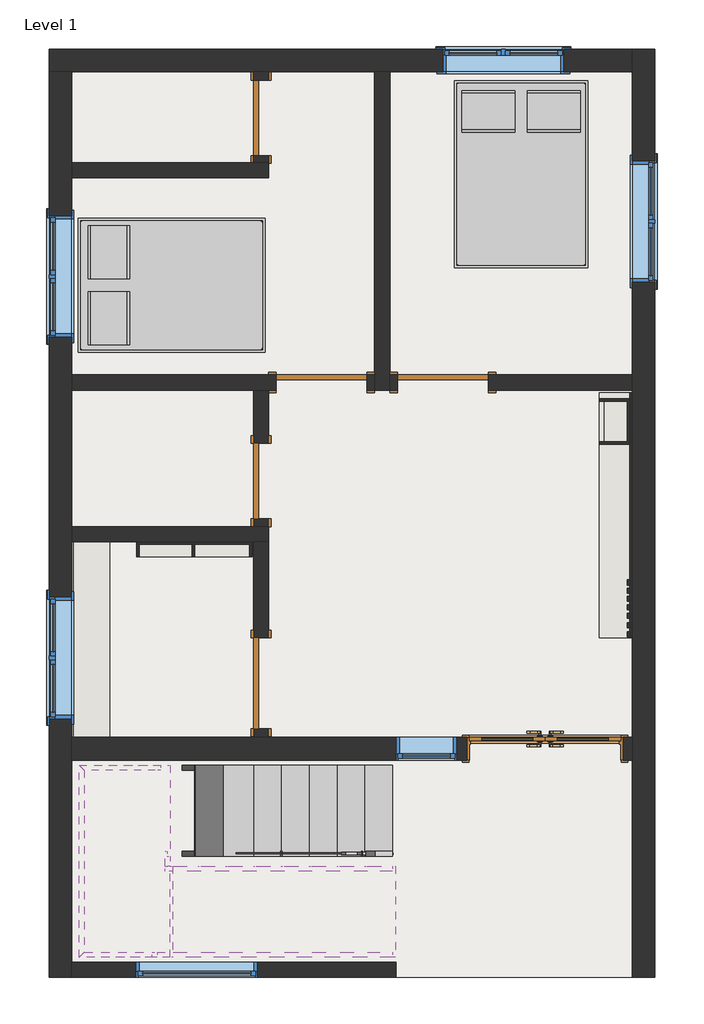
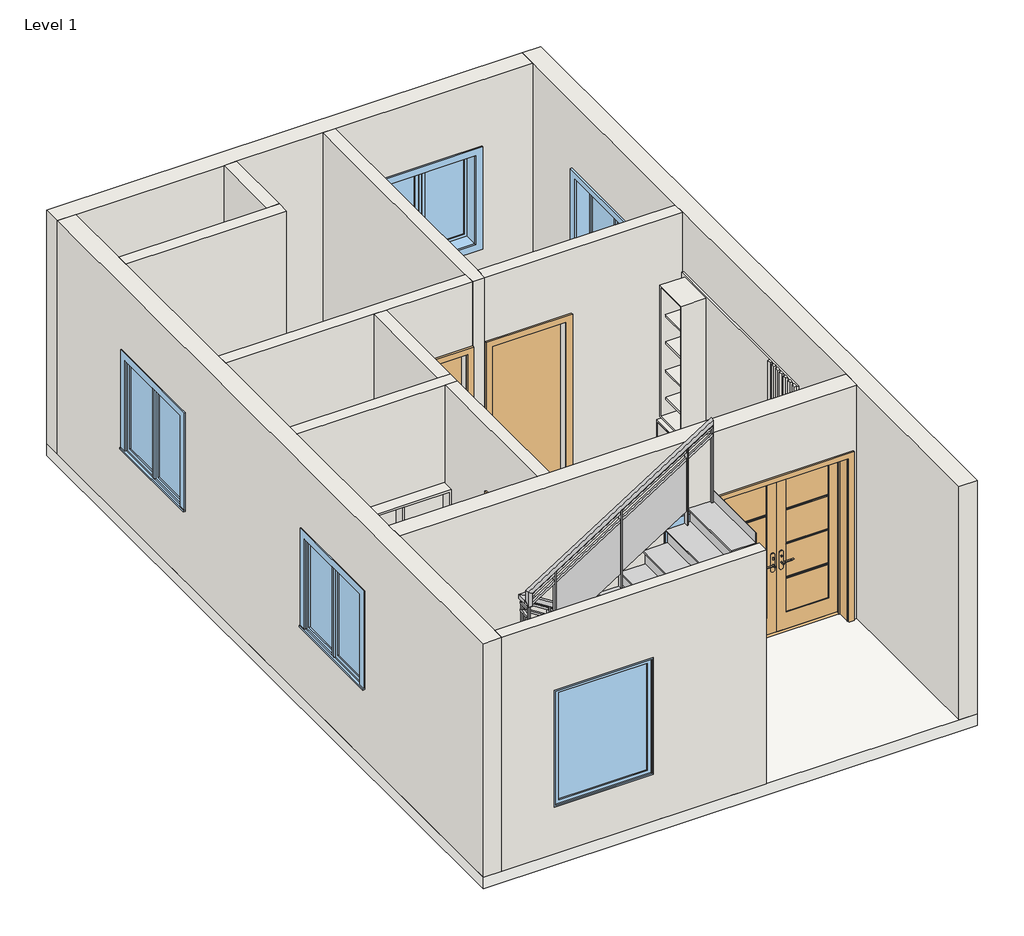
# One storey: 15 walls, 8 members, 6 doors, 6 windows, 2 furniture elements, 2 slabs, 2 stair flights, 1 railing.
# Revit data of these elements (continued)
# Element 41 (IfcWindow, "Fixed : 24\" x 72\"") (continued)
#   Phase Created = New Construction
#   Materials on its faces: "Sash", "Glass"
# Element 42 (IfcWindow, "Fixed : 4'")
#   Mark = "15"
#   Phase Created = New Construction
#   Materials on its faces: "Sash", "Glass"
# Materials
#   "Cherry": class "Wood", colour RGB 226 177 128, transparency 0, Description = "Prunus Serotina", Cost = 0
#   "Glass": class "Glass", colour RGB 0 128 192, transparency 0.75, Description = "Soda Lime Glass", Cost = 0
#   "Aluminum": class "Metal", colour RGB 247 247 247, transparency 0, Description = "Aluminum 6061", Cost = 0
#   "Door - Panel": class "Wood", colour RGB 210 159 95, transparency 0
#   "Door - Frame": colour RGB 118 70 51, transparency 0
#   "Birch": class "Wood", colour RGB 224 178 126, transparency 0, Description = "Betula Alleghaniensis", Cost = 0
#   "Linen, White": class "Textile", colour RGB 247 247 239, transparency 0, Description = "Linen, white", Cost = 0
#   "floor": class "Generic", colour RGB 138 129 123, transparency 0, Cost = 0
#   "ext wall": class "Generic", colour RGB 219 210 180, transparency 0, Cost = 0
#   "int wall": class "Generic", colour RGB 230 213 172, transparency 0, Cost = 0
#   "Sash": class "Wood", colour RGB 224 178 126, transparency 0
#   "Trim": class "Wood", colour RGB 224 178 126, transparency 0
#   "drawers": class "Generic", colour RGB 121 66 39, transparency 0, Cost = 0
#   "wood": class "Generic", colour RGB 255 226 181, transparency 0, Cost = 0
#   "clear glass": class "Generic", colour RGB 141 181 235, transparency 0.9, Cost = 0
#   "stone": class "Generic", colour RGB 125 126 130, transparency 0, Cost = 0
#   "Default Wall": colour RGB 128 128 128, transparency 0
#   "metal": class "Generic", colour RGB 76 25 7, transparency 0, Cost = 0
